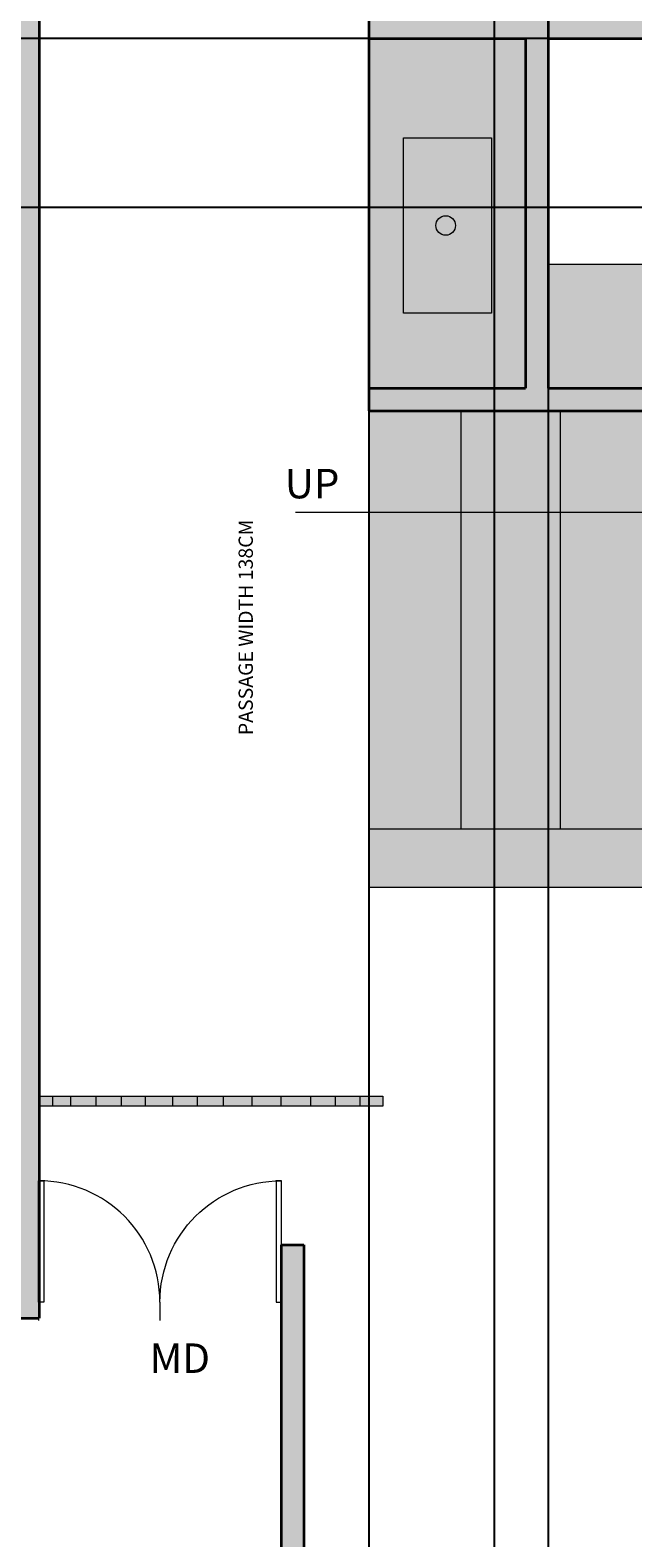
# Model space of a CAD drawing. Units: inches. Extents: x 192 to 1361, y -1362 to 367.
# Tile 11 of 23: x 649 to 891, y -1057 to -454. Entities that reach past the tile are written whole.
import ezdxf

# ---------------------------------------------------------------- set-up
doc = ezdxf.new("R2010")
doc.units = ezdxf.units.IN
doc.header["$MEASUREMENT"] = 0
for name, color, linetype, lineweight in [('A-ANNO-DIMS', 2, 'Continuous', 18), ('A-ANNO-SYMB', 7, 'Continuous', 18), ('A-DOOR', 4, 'Continuous', 18), ('A-FLOR-CASE', 32, 'Continuous', 18), ('A-FLOR-FIXT', 8, 'Continuous', 18), ('A-FLOR-PRTN', 32, 'Continuous', 18), ('A-FLOR-PRTN-PATT', 32, 'Continuous', 13), ('A-FLOR-STRS', 7, 'Continuous', 18), ('A-WALL-PATT', 250, 'Continuous', 13), ('text', 7, 'Continuous', 18), ('walls', 7, 'Continuous', 35)]:
    doc.layers.add(name, color=color, linetype=linetype, lineweight=lineweight)
doc.layers.add('A-FLOR-CASE-PATT', color=9, linetype='Continuous', lineweight=13, true_color=0xc7c8ca)
doc.layers.add('A-FLOR-STRS-PATT', color=252, linetype='Continuous', lineweight=13, true_color=0x939598)
doc.styles.get("Standard").update_dxf_attribs({"font": 'arial.ttf'})
doc.dimstyles.get("Standard").update_dxf_attribs({"dimtxt": 0.18, "dimasz": 0.18, "dimexe": 0.18, "dimexo": 0.0625, "dimgap": 0.09, "dimtad": 0, "dimtih": 1, "dimtoh": 1, "dimzin": 0, "dimdsep": 46, "dimlunit": 3, "dimtxsty": 'Standard', "dimcen": 0.09, "dimadec": 0, "dimazin": 0, "dimtfac": 1, "dimtofl": 0, "dimtmove": 0, "dimatfit": 3, "dimfxl": 1, "dimtolj": 1, "dimtzin": 0, "dimarcsym": 0})

# ---------------------------------------------------------------- blocks, each defined once
blk = doc.blocks.new('*U2')
for p, q in [((0, 0), (0, -6)), ((40, 0), (40, -6))]:
    blk.add_line(p, q)
blk.add_lwpolyline([(0, 0), (0, 40), (1.75, 40), (1.75, 0)], close=True)
blk.add_arc((0, 0), 40, 0, 90)
blk = doc.blocks.new('*D47')
at = {"layer": 'A-ANNO-DIMS', "color": 0, "lineweight": -2, "transparency": 16777216}
for p, q in [((1273.57, -782.95), (1273.57, -1200.05)), ((274.89, -914.5), (274.89, -1200.05)), ((275.07, -1199.87), (773.84, -1199.87)), ((1273.39, -1199.87), (774.62, -1199.87))]:
    blk.add_line(p, q, dxfattribs=at)
at = {"layer": 'A-ANNO-DIMS', "color": 0, "transparency": 16777216}
for points in [[(275.07, -1199.84), (275.07, -1199.9), (274.89, -1199.87)], [(1273.39, -1199.84), (1273.39, -1199.9), (1273.57, -1199.87)]]:
    blk.add_solid(points, dxfattribs=at)
at = {"layer": 'Defpoints', "color": 0, "transparency": 16777216}
for p in [(1273.57, -782.89), (274.89, -914.44), (1273.57, -1199.87)]:
    blk.add_point(p, dxfattribs=at)
at = {"layer": 'A-ANNO-DIMS', "color": 0, "transparency": 16777216, "insert": (774.23, -1199.87), "char_height": 0.18, "attachment_point": 5}
blk.add_mtext('\\A1;998.7', dxfattribs=at)
blk = doc.blocks.new('*D67')
at = {"layer": 'A-ANNO-DIMS', "color": 0, "lineweight": -2, "transparency": 16777216}
for p, q in [((784.8, -597.56), (784.8, -1200.05)), ((856.57, -597.56), (856.57, -1200.05)), ((784.98, -1199.87), (820.29, -1199.87)), ((856.39, -1199.87), (821.08, -1199.87))]:
    blk.add_line(p, q, dxfattribs=at)
at = {"layer": 'A-ANNO-DIMS', "color": 0, "transparency": 16777216}
for points in [[(784.98, -1199.84), (784.98, -1199.9), (784.8, -1199.87)], [(856.39, -1199.84), (856.39, -1199.9), (856.57, -1199.87)]]:
    blk.add_solid(points, dxfattribs=at)
at = {"layer": 'Defpoints', "color": 0, "transparency": 16777216}
for p in [(784.8, -597.5), (856.57, -597.5), (856.57, -1199.87)]:
    blk.add_point(p, dxfattribs=at)
at = {"layer": 'A-ANNO-DIMS', "color": 0, "transparency": 16777216, "insert": (820.69, -1199.87), "char_height": 0.18, "attachment_point": 5}
blk.add_mtext('\\A1;71.76', dxfattribs=at)
blk = doc.blocks.new('*D68')
at = {"layer": 'A-ANNO-DIMS', "color": 0, "lineweight": -2, "transparency": 16777216}
for p, q in [((856.57, -597.56), (856.57, -1200.05)), ((971.58, -597.56), (971.58, -1200.05)), ((856.75, -1199.87), (913.79, -1199.87)), ((971.4, -1199.87), (914.36, -1199.87))]:
    blk.add_line(p, q, dxfattribs=at)
at = {"layer": 'A-ANNO-DIMS', "color": 0, "transparency": 16777216}
for points in [[(856.75, -1199.84), (856.75, -1199.9), (856.57, -1199.87)], [(971.4, -1199.84), (971.4, -1199.9), (971.58, -1199.87)]]:
    blk.add_solid(points, dxfattribs=at)
at = {"layer": 'Defpoints', "color": 0, "transparency": 16777216}
for p in [(856.57, -597.5), (971.58, -597.5), (971.58, -1199.87)]:
    blk.add_point(p, dxfattribs=at)
at = {"layer": 'A-ANNO-DIMS', "color": 0, "transparency": 16777216, "insert": (914.07, -1199.87), "char_height": 0.18, "attachment_point": 5}
blk.add_mtext('\\A1;115', dxfattribs=at)
blk = doc.blocks.new('*D69')
at = {"layer": 'A-ANNO-DIMS', "color": 0, "lineweight": -2, "transparency": 16777216}
for p, q in [((981.75, -457.5), (192.16, -457.5)), ((192.34, -457.68), (192.34, -491.13)), ((192.34, -524.95), (192.34, -491.5)), ((980.52, -525.13), (192.16, -525.13))]:
    blk.add_line(p, q, dxfattribs=at)
at = {"layer": 'A-ANNO-DIMS', "color": 0, "transparency": 16777216}
for points in [[(192.31, -457.68), (192.37, -457.68), (192.34, -457.5)], [(192.31, -524.95), (192.37, -524.95), (192.34, -525.13)]]:
    blk.add_solid(points, dxfattribs=at)
at = {"layer": 'Defpoints', "color": 0, "transparency": 16777216}
for p in [(981.81, -457.5), (192.34, -525.13), (980.58, -525.13)]:
    blk.add_point(p, dxfattribs=at)
at = {"layer": 'A-ANNO-DIMS', "color": 0, "transparency": 16777216, "insert": (192.34, -491.31), "char_height": 0.18, "attachment_point": 5}
blk.add_mtext('\\A1;67.63', dxfattribs=at)
blk = doc.blocks.new('*D72')
at = {"layer": 'A-ANNO-DIMS', "color": 0, "lineweight": -2, "transparency": 16777216}
for p, q in [((835.08, -1067.56), (835.08, 367.39)), ((835.26, 367.21), (935.95, 367.21)), ((1037.58, 367.21), (936.88, 367.21)), ((1037.76, -1067.56), (1037.76, 367.39))]:
    blk.add_line(p, q, dxfattribs=at)
at = {"layer": 'A-ANNO-DIMS', "color": 0, "transparency": 16777216}
for points in [[(835.26, 367.24), (835.26, 367.18), (835.08, 367.21)], [(1037.58, 367.24), (1037.58, 367.18), (1037.76, 367.21)]]:
    blk.add_solid(points, dxfattribs=at)
at = {"layer": 'Defpoints', "color": 0, "transparency": 16777216}
for p in [(1037.76, 367.21), (835.08, -1067.62), (1037.76, -1067.62)]:
    blk.add_point(p, dxfattribs=at)
at = {"layer": 'A-ANNO-DIMS', "color": 0, "transparency": 16777216, "insert": (936.42, 367.21), "char_height": 0.18, "attachment_point": 5}
blk.add_mtext('\\A1;202.68', dxfattribs=at)

msp = doc.modelspace()

# ---------------------------------------------------------------- hatches: boundary and pattern name
at = {"layer": 'A-FLOR-CASE-PATT'}
h = msp.add_hatch(color=256, dxfattribs=at)
h.dxf.hatch_style = 1
h.paths.add_polyline_path([(831.9452, -487.1432), (796.7394, -487.1432), (796.7394, -557.2159), (831.9452, -557.2159)], flags=0)
h.paths.add_polyline_path([(817.5051, -522.1795, -1), (809.6555, -522.1795, -1)], flags=0)
h.paths.add_polyline_path([(847.5691, -457.4996), (784.8041, -457.4996), (784.8041, -597.4996), (847.5691, -597.4996)])
h.paths.add_polyline_path([(831.9452, -487.1432), (831.9452, -557.2159), (796.7394, -557.2159), (796.7394, -487.1432)], flags=16)
h = msp.add_hatch(color=256, dxfattribs=at)
h.dxf.hatch_style = 1
h.paths.add_polyline_path([(847.5691, -457.4996), (784.8041, -457.4996), (784.8041, -597.4996), (847.5691, -597.4996)])
h = msp.add_hatch(color=256, dxfattribs=at)
h.dxf.hatch_style = 1
h.paths.add_polyline_path([(971.5799, -548.0101), (856.5691, -548.0101), (856.5691, -597.4996), (971.5799, -597.4996)])
h = msp.add_hatch(color=256, dxfattribs=at)
h.dxf.hatch_style = 1
h.paths.add_polyline_path([(1099.8366, -773.892), (784.8041, -773.892), (784.8041, -797.1415), (1099.8366, -797.1415)])
at = {"layer": 'A-FLOR-PRTN-PATT'}
h = msp.add_hatch(color=256, dxfattribs=at)
h.dxf.hatch_style = 1
h.paths.add_polyline_path([(658.1969, -880.6608), (652.8925, -880.6608), (652.8925, -884.7084), (658.1969, -884.7084)])
h.paths.add_polyline_path([(675.6194, -880.6608), (665.4441, -880.6608), (665.4441, -884.7084), (675.6194, -884.7084)])
h.paths.add_polyline_path([(695.3294, -880.6608), (685.7481, -880.6608), (685.7481, -884.7084), (695.3294, -884.7084)])
h.paths.add_polyline_path([(716.1382, -880.6608), (706.2513, -880.6608), (706.2513, -884.7084), (716.1382, -884.7084)])
h.paths.add_polyline_path([(737.9964, -880.6608), (726.476, -880.6608), (726.476, -884.7084), (737.9964, -884.7084)])
h.paths.add_polyline_path([(761.5242, -880.6608), (749.5916, -880.6608), (749.5916, -884.7084), (761.5242, -884.7084)])
h.paths.add_polyline_path([(781.2244, -880.6608), (771.3506, -880.6608), (771.3506, -884.7084), (781.2244, -884.7084)])
h = msp.add_hatch(color=256, dxfattribs=at)
h.dxf.hatch_style = 1
h.paths.add_polyline_path([(665.4441, -880.6608), (658.1969, -880.6608), (658.1969, -884.7084), (665.4441, -884.7084)])
h.paths.add_polyline_path([(685.7481, -880.6608), (675.6194, -880.6608), (675.6194, -884.7084), (685.7481, -884.7084)])
h.paths.add_polyline_path([(706.2513, -880.6608), (695.3294, -880.6608), (695.3294, -884.7084), (706.2513, -884.7084)])
h.paths.add_polyline_path([(726.476, -880.6608), (716.1382, -880.6608), (716.1382, -884.7084), (726.476, -884.7084)])
h.paths.add_polyline_path([(749.5916, -880.6608), (737.9964, -880.6608), (737.9964, -884.7084), (749.5916, -884.7084)])
h.paths.add_polyline_path([(771.3506, -880.6608), (761.5242, -880.6608), (761.5242, -884.7084), (771.3506, -884.7084)])
h.paths.add_polyline_path([(790.5088, -880.6608), (781.2244, -880.6608), (781.2244, -884.7084), (790.5088, -884.7084)])
at = {"layer": 'A-FLOR-STRS-PATT'}
h = msp.add_hatch(color=256, dxfattribs=at)
h.dxf.hatch_style = 1
h.paths.add_polyline_path([(821.7257, -606.4996), (784.8041, -606.4996), (784.8041, -773.892), (821.7257, -773.892)])
h.paths.add_polyline_path([(861.4265, -606.4996), (821.7257, -606.4996), (821.7257, -773.892), (861.4265, -773.892)])
h.paths.add_polyline_path([(940.828, -606.4996), (901.1272, -606.4996), (901.1272, -773.892), (940.828, -773.892)])
h.paths.add_polyline_path([(901.1272, -606.4996), (861.4265, -606.4996), (861.4265, -773.892), (901.1272, -773.892)])
h.paths.add_polyline_path([(980.5288, -687.5154), (980.5288, -606.4996), (940.828, -606.4996), (940.828, -773.892), (980.5288, -773.892)])
h.paths.add_polyline_path([(1020.2295, -606.4996), (980.5288, -606.4996), (980.5288, -687.5154), (1020.2295, -687.5154)])
h.paths.add_polyline_path([(1059.9303, -606.4996), (1020.2295, -606.4996), (1020.2295, -687.5154), (1059.9303, -687.5154)])
h.paths.add_polyline_path([(1099.631, -606.4996), (1059.9303, -606.4996), (1059.9303, -687.5154), (1076.4416, -687.5154), (1099.631, -687.5154)])
h.paths.add_polyline_path([(1139.3318, -606.4996), (1099.631, -606.4996), (1099.631, -687.5154), (1139.3318, -687.5154)])
h.paths.add_polyline_path([(1177.0582, -606.4996), (1139.3318, -606.4996), (1139.3318, -687.5154), (1177.0582, -687.5154)])
h.paths.add_polyline_path([(1264.5658, -606.4996), (1177.0582, -606.4996), (1177.0582, -687.5154), (1177.0582, -773.892), (1264.5658, -773.892)])
at = {"layer": 'A-WALL-PATT'}
h = msp.add_hatch(color=256, dxfattribs=at)
h.dxf.hatch_style = 1
h.paths.add_polyline_path([(309.5452, 191.102), (300.5452, 191.102), (300.5452, -126.898), (309.5452, -126.898), (309.5452, -117.898)])
h.paths.add_polyline_path([(420.798, 191.102), (337.3229, 191.102), (337.3229, 182.102), (420.798, 182.102)])
h.paths.add_polyline_path([(518.5452, 182.102), (625.4022, 182.102), (625.4022, 191.102), (509.5452, 191.102), (509.5452, 114.3262), (518.5452, 114.3262)])
h.paths.add_polyline_path([(842.5452, 191.102), (763.4438, 191.102), (763.4438, 182.102), (833.5452, 182.102), (833.5452, 161.1615), (836.8088, 161.1615), (842.5452, 161.1615)])
h.paths.add_polyline_path([(842.5452, -16.5675), (833.5452, -16.5675), (833.5452, -60.4996), (784.8041, -60.4996), (784.8041, -354.6796), (793.8041, -354.6796), (793.8041, -69.4996), (1094.1252, -69.4996), (1094.1252, -60.4996), (842.5452, -60.4996)])
h.paths.add_polyline_path([(518.5452, 36.602), (509.5452, 36.602), (509.5452, -117.898), (420.2204, -117.898), (420.2204, -126.898), (518.5452, -126.898)])
h.paths.add_polyline_path([(474.8041, -377.0384), (465.8041, -377.0384), (465.8041, -381.5384), (465.8041, -450.898), (537.5717, -450.898), (537.5717, -441.898), (474.8041, -441.898)])
h.paths.add_polyline_path([(1162.8041, -380.6763), (1204.3001, -380.6763), (1204.3001, -375.6763), (1195.1471, -375.6763), (1153.8041, -375.6763), (1153.8041, -448.4996), (856.5691, -448.4996), (856.5691, -457.4996), (1162.8041, -457.4996)])
h.paths.add_polyline_path([(1162.8041, -525.128), (1153.8041, -525.128), (1153.8041, -597.4996), (1162.8041, -597.4996)], flags=17)
h.paths.add_polyline_path([(1162.8041, -60.4996), (1153.8041, -60.4996), (1153.8041, -69.4996), (1153.8041, -177.4733), (1205.8889, -177.4733), (1205.8889, -172.4733), (1162.8041, -172.4733)])
h.paths.add_polyline_path([(980.5799, -525.686), (971.5799, -525.686), (971.5799, -597.4996), (980.5799, -597.4996)], flags=17)
h.paths.add_polyline_path([(856.5691, -448.4996), (798.7542, -448.4996), (784.8041, -448.4996), (784.8041, -457.4996), (847.5691, -457.4996), (847.5691, -597.4996), (784.8041, -597.4996), (784.8041, -606.4996), (1273.5658, -606.4996), (1273.5658, -597.4996), (856.5691, -597.4996)])
h.paths.add_polyline_path([(1273.5658, -773.892), (1099.8366, -773.892), (1099.8366, -851.9362), (1108.8366, -851.9362), (1108.8366, -782.892), (1273.5658, -782.892)])
h.paths.add_polyline_path([(1108.8366, -982.9214), (1099.8366, -982.9214), (1099.8366, -1067.6246), (1037.7563, -1067.6246), (1037.7563, -1076.6246), (1108.8366, -1076.6246)])
h.paths.add_polyline_path([(835.078, -1067.6246), (758.8458, -1067.6246), (758.8458, -940.2324), (749.8458, -940.2324), (749.8458, -963.172), (749.8458, -970.4644), (749.8458, -1076.6246), (835.078, -1076.6246)])
h.paths.add_polyline_path([(450.307, -1066.9838), (441.307, -1066.9838), (441.307, -1076.6246), (450.307, -1076.6246)])
h.paths.add_polyline_path([(492.8925, -756.4415), (274.8925, -756.4415), (274.8925, -765.4415), (492.8925, -765.4415)])
h.paths.add_polyline_path([(283.8925, -835.2244), (274.8925, -835.2244), (274.8925, -914.4415), (492.8925, -914.4415), (492.8925, -839.9415), (483.8925, -839.9415), (483.8925, -905.4415), (283.8925, -905.4415)])
h.paths.add_polyline_path([(283.8925, -441.898), (283.8925, -375.4296), (281.6021, -375.4296), (281.6021, -399.4121), (274.8925, -399.4121), (274.8925, -441.898), (274.8925, -684.5089), (283.8925, -684.5089)])
h = msp.add_hatch(color=256, dxfattribs=at)
h.dxf.hatch_style = 1
h.paths.add_polyline_path([(652.8925, -441.898), (643.8925, -441.898), (643.8925, -457.8461), (643.8925, -564.167), (643.8925, -905.4415), (578.0245, -905.4415), (578.0245, -914.4415), (643.8925, -914.4415), (643.8925, -969.5484), (652.6138, -969.5484), (652.6138, -963.172), (652.6138, -914.556)])
h.paths.add_polyline_path([(509.5452, 191.102), (504.3983, 191.102), (504.3983, 182.102), (509.5452, 182.102)])

# ---------------------------------------------------------------- linework, layer by layer
at = {"layer": 'A-ANNO-SYMB'}
msp.add_line((755.4527, -647.0075), (1219.7014, -647.0075), dxfattribs=at)
at = {"layer": 'A-FLOR-CASE'}
for p, q in [((971.5799, -548.0101), (856.5691, -548.0101)), ((1099.8366, -773.892), (784.8041, -773.892)), ((784.8041, -773.892), (784.8041, -797.1415)), ((784.8041, -784.892), (784.8041, -786.892)), ((784.8041, -797.1415), (1099.8366, -797.1415))]:
    msp.add_line(p, q, dxfattribs=at)
at = {"layer": 'A-FLOR-FIXT'}
for p, q in [((798.7649, -497.318), (833.9707, -497.318)), ((798.7649, -567.3907), (798.7649, -497.318)), ((833.9707, -497.318), (833.9707, -567.3907)), ((833.9707, -567.3907), (798.7649, -567.3907))]:
    msp.add_line(p, q, dxfattribs=at)
msp.add_circle((815.6058, -532.3543), 3.9248, dxfattribs=at)
at = {"layer": 'A-FLOR-PRTN'}
for p, q in [((652.8925, -880.6608), (790.5088, -880.6608)), ((658.1969, -880.6608), (658.1969, -884.7084)), ((665.4441, -880.6608), (665.4441, -884.7084)), ((675.6194, -880.6608), (675.6194, -884.7084)), ((685.7481, -880.6608), (685.7481, -884.7084)), ((695.3294, -880.6608), (695.3294, -884.7084)), ((706.2513, -880.6608), (706.2513, -884.7084)), ((716.1382, -880.6608), (716.1382, -884.7084)), ((726.476, -880.6608), (726.476, -884.7084)), ((737.9964, -880.6608), (737.9964, -884.7084)), ((749.5916, -880.6608), (749.5916, -884.7084)), ((761.5242, -880.6608), (761.5242, -884.7084)), ((771.3506, -880.6608), (771.3506, -884.7084)), ((781.2244, -880.6608), (781.2244, -884.7084)), ((790.5088, -880.6608), (790.5088, -884.7084)), ((790.5088, -884.7084), (652.8925, -884.7084))]:
    msp.add_line(p, q, dxfattribs=at)
at = {"layer": 'A-FLOR-STRS'}
for p, q in [((784.8041, -606.4996), (784.8041, -773.892)), ((784.8041, -606.4996), (784.8041, -773.892)), ((821.7257, -606.4996), (821.7257, -773.892)), ((821.7257, -606.4996), (821.7257, -773.892)), ((861.4265, -606.4996), (861.4265, -773.892)), ((861.4265, -606.4996), (861.4265, -773.892))]:
    msp.add_line(p, q, dxfattribs=at)
at = {"layer": 'walls'}
for p, q in [((652.8925, -441.898), (652.8925, -969.5484)), ((784.8041, -448.4996), (784.8041, -606.4996)), ((856.5691, -448.4996), (856.5691, -597.4996)), ((784.8041, -457.4996), (847.5691, -457.4996)), ((847.5691, -457.4996), (847.5691, -597.4996)), ((856.5691, -457.4996), (1162.8041, -457.4996)), ((784.8041, -597.4996), (847.5691, -597.4996)), ((856.5691, -597.4996), (1273.5658, -597.4996)), ((784.8041, -606.4996), (1273.5658, -606.4996)), ((749.8458, -1076.6246), (749.8458, -940.2324)), ((749.8458, -940.2324), (758.8458, -940.2324)), ((758.8458, -940.2324), (758.8458, -1067.6246)), ((643.8925, -969.5484), (652.8925, -969.5484))]:
    msp.add_line(p, q, dxfattribs=at)

# ---------------------------------------------------------------- block references
at = {"layer": 'A-DOOR', "yscale": 1.215399430198434, "zscale": 1.215399430198434}
for p, xscale in [((652.6138, -963.172), 1.215399430198434), ((749.8458, -963.172), -1.215399430198434)]:
    msp.add_blockref('*U2', p, dxfattribs=dict(at, xscale=xscale))

# ---------------------------------------------------------------- texts
at = {"layer": 'A-ANNO-SYMB'}
msp.add_text('UP', height=11.81288, dxfattribs=at).set_placement((751.2125, -641.5317))
at = {"layer": 'text'}
msp.add_text('PASSAGE WIDTH 138CM', height=5.711952, rotation=90, dxfattribs=at).set_placement((738.427, -736.2757))
msp.add_text('MD', height=11.81288, dxfattribs=at).set_placement((697.1156, -991.4601))

# ---------------------------------------------------------------- dimensions: what is measured, and where the dimension line sits
at = {"layer": 'A-ANNO-DIMS'}
for base, p1, p2, override, picture, middle in [((1037.7563, 367.2097), (835.078, -1067.6246), (1037.7563, -1067.6246), {"dimdec": 2, "dimlfac": 1, "dimrnd": 0, "dimzin": 0, "dimdsep": 46, "dimlunit": 2}, '*D72', (936.4171, 367.2097)), ((856.56907, -1199.87271), (784.80414, -597.49959), (856.56907, -597.49959), {"dimdec": 2, "dimlfac": 1, "dimrnd": 0, "dimzin": 0, "dimdsep": 46, "dimlunit": 2}, '*D67', (820.68661, -1199.87271)), ((971.5799, -1199.8727), (856.5691, -597.4996), (971.5799, -597.4996), {"dimdec": 0, "dimlfac": 1, "dimrnd": 0, "dimzin": 0, "dimdsep": 46, "dimlunit": 2}, '*D68', (914.0745, -1199.8727)), ((1273.5658, -1199.8727), (274.8925, -914.4415), (1273.5658, -782.892), {"dimdec": 1, "dimlfac": 1, "dimrnd": 0, "dimzin": 0, "dimdsep": 46, "dimlunit": 2}, '*D47', (774.2292, -1199.8727))]:
    dim = msp.add_linear_dim(base=base, p1=p1, p2=p2, dimstyle='Standard', override=override, dxfattribs=at)
    dim.commit()
    dim.dimension.update_dxf_attribs({"geometry": picture, "text_midpoint": middle})
dim = msp.add_linear_dim(base=(192.3425, -525.128), p1=(981.8078, -457.4996), p2=(980.5799, -525.128), angle=90, dimstyle='Standard', override={"dimdec": 2, "dimlfac": 1, "dimrnd": 0, "dimzin": 0, "dimdsep": 46, "dimlunit": 2}, dxfattribs=at)
dim.commit()
dim.dimension.update_dxf_attribs({"geometry": '*D69', "text_midpoint": (192.3425, -491.3138)})

doc.saveas('drawing.dxf')
